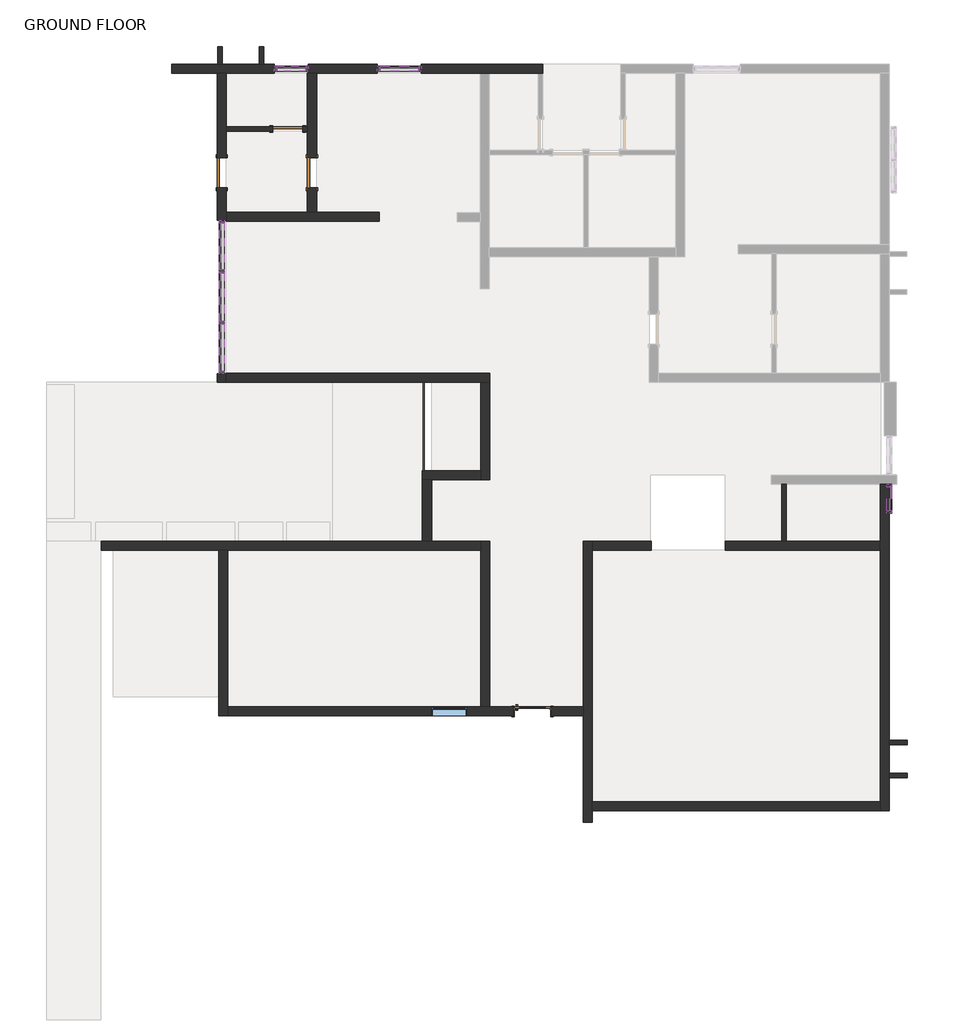
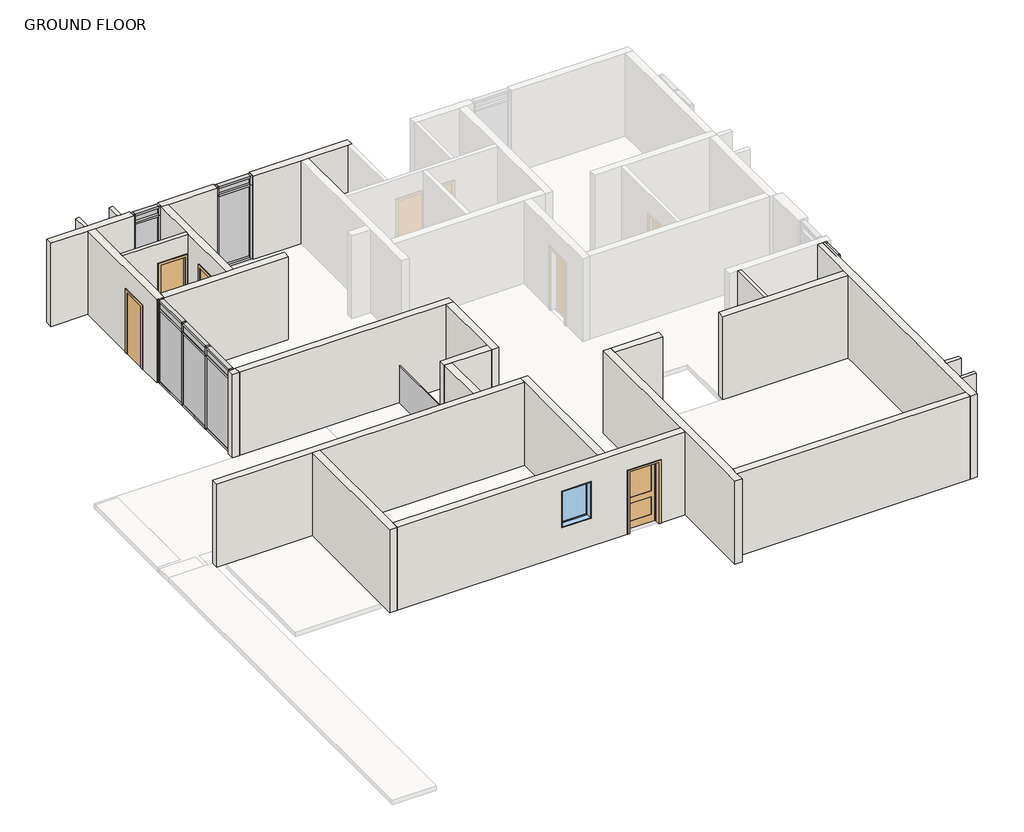
# One storey, part 1 of 2: 38 members, 23 walls, 13 plates, 4 doors, 1 window.
"""IFC4 building model written with IfcOpenShell, lengths in millimetres."""

from ifc_helpers import new_model, si_unit, frame, origin, place, context, project, spatial, polyline, outline, extrude, faceted_brep, transform, mapped, element, save
from components import door_18b56f29, door_f2b275c1, door_85036156, member_3e1bda4a, member_b6df92ca, member_34ede31c, member_a972b4dd, member_f0fea5a5, member_75d1e245, member_ee409385, member_3c3dc66a, member_8f63b531, member_3b0b2d0d, member_d7af48b5, member_8ca7f02a, member_47bfaf8a, member_6e77e263, system_panel_glazed_33731b62, system_panel_glazed_44b51bf5, system_panel_glazed_4e629a68, system_panel_glazed_8059ee36, system_panel_glazed_a992b757, system_panel_glazed_7419534f, system_panel_glazed_091cc013, system_panel_glazed_6c905176, system_panel_glazed_bc4b8a1a, system_panel_glazed_9fd37d83, system_panel_glazed_bf88fd99, window_c1f32544

model = new_model("IFC4")

# Units and contexts
model_context = context("Model", 3, world=origin())
ifc_project = project(units=[si_unit("LENGTHUNIT", "METRE", prefix="MILLI")], contexts=[model_context])

# Site, building, storey
site = spatial("IfcSite", under=ifc_project)
building = spatial("IfcBuilding", under=site)
storey = spatial("IfcBuildingStorey", under=building, Name="GROUND FLOOR", Elevation=304.8)

# Doors
placement = place(None, origin())
door_shape = door_18b56f29(model_context)
element("IfcDoor", 1, ObjectType="Door-Interior-Single-2_Panel-Wood : 36\" x 80\"", at=placement, inside=storey, context=model_context, shape_type="MappedRepresentation", body=[
    mapped(door_shape, transform((2388.7237558, 174.0966143, 304.8), x_axis=(1.0, 0.0, 0.0), y_axis=(0.0, 1.0, 0.0), z_axis=(0.0, 0.0, 1.0))),
])
door_2_shape = door_f2b275c1(model_context)
element("IfcDoor", 2, ObjectType="Single-Flush : 30\" x 80\"", at=placement, inside=storey, context=model_context, shape_type="MappedRepresentation", body=[
    mapped(door_2_shape, transform((-3801.944009, 14911.54348, 304.8), x_axis=(-1.0, 0.0, 0.0), y_axis=(0.0, -1.0, 0.0), z_axis=(0.0, 0.0, 1.0))),
])
door_3_shape = door_85036156(model_context)
element("IfcDoor", 3, ObjectType="Single-Flush : 30\" x 80\"", at=placement, inside=storey, context=model_context, shape_type="MappedRepresentation", body=[
    mapped(door_3_shape, transform((-3192.344009, 13803.0266219, 304.8), x_axis=(0.0, -1.0, 0.0), y_axis=(1.0, 0.0, 0.0), z_axis=(0.0, 0.0, 1.0))),
])
element("IfcDoor", 4, ObjectType="Single-Flush : 30\" x 80\"", at=placement, inside=storey, context=model_context, shape_type="MappedRepresentation", body=[
    mapped(door_3_shape, transform((-5478.344009, 13803.0266219, 304.8), x_axis=(0.0, -1.0, 0.0), y_axis=(1.0, 0.0, 0.0), z_axis=(0.0, 0.0, 1.0))),
])

# Members
member_shape = member_3e1bda4a(model_context)
element("IfcMember", 5, ObjectType="Rectangular Mullion : 2.5\" x 5\" rectangular", at=placement, inside=storey, context=model_context, shape_type="MappedRepresentation", body=[
    mapped(member_shape, transform((-5478.344009, 12544.7356247, 3048.0), x_axis=(0.0, 0.0, 1.0), y_axis=(1.0, 0.0, 0.0), z_axis=(0.0, 1.0, 0.0))),
])
element("IfcMember", 6, ObjectType="Rectangular Mullion : 2.5\" x 5\" rectangular", at=placement, inside=storey, context=model_context, shape_type="MappedRepresentation", body=[
    mapped(member_shape, transform((-5478.344009, 9985.6856249, 3048.0), x_axis=(0.0, 0.0, 1.0), y_axis=(1.0, 0.0, 0.0), z_axis=(0.0, 1.0, 0.0))),
])
member_2_shape = member_b6df92ca(model_context)
element("IfcMember", 7, ObjectType="Rectangular Mullion : 2.5\" x 5\" rectangular", at=placement, inside=storey, context=model_context, shape_type="MappedRepresentation", body=[
    mapped(member_2_shape, transform((-5478.344009, 11281.0856246, 3048.0), x_axis=(0.0, 0.0, 1.0), y_axis=(1.0, 0.0, 0.0), z_axis=(0.0, 1.0, 0.0))),
])
element("IfcMember", 8, ObjectType="Rectangular Mullion : 2.5\" x 5\" rectangular", at=placement, inside=storey, context=model_context, shape_type="MappedRepresentation", body=[
    mapped(member_shape, transform((-5478.344009, 8785.5356247, 304.8), x_axis=(0.0, 0.0, -1.0), y_axis=(1.0, 0.0, 0.0), z_axis=(0.0, -1.0, 0.0))),
])
element("IfcMember", 9, ObjectType="Rectangular Mullion : 2.5\" x 5\" rectangular", at=placement, inside=storey, context=model_context, shape_type="MappedRepresentation", body=[
    mapped(member_shape, transform((-5478.344009, 11344.5856246, 304.8), x_axis=(0.0, 0.0, -1.0), y_axis=(1.0, 0.0, 0.0), z_axis=(0.0, -1.0, 0.0))),
])
element("IfcMember", 10, ObjectType="Rectangular Mullion : 2.5\" x 5\" rectangular", at=placement, inside=storey, context=model_context, shape_type="MappedRepresentation", body=[
    mapped(member_2_shape, transform((-5478.344009, 10049.1856249, 304.8), x_axis=(0.0, 0.0, -1.0), y_axis=(1.0, 0.0, 0.0), z_axis=(0.0, -1.0, 0.0))),
])
member_3_shape = member_34ede31c(model_context)
element("IfcMember", 11, ObjectType="Rectangular Mullion : 2.5\" x 5\" rectangular", at=placement, inside=storey, context=model_context, shape_type="MappedRepresentation", body=[
    mapped(member_3_shape, transform((-5478.344009, 9985.6856249, 2743.2), x_axis=(0.0, 0.0, 1.0), y_axis=(1.0, 0.0, 0.0), z_axis=(0.0, 1.0, 0.0))),
])
element("IfcMember", 12, ObjectType="Rectangular Mullion : 2.5\" x 5\" rectangular", at=placement, inside=storey, context=model_context, shape_type="MappedRepresentation", body=[
    mapped(member_3_shape, transform((-5478.344009, 12544.7356247, 2743.2), x_axis=(0.0, 0.0, 1.0), y_axis=(1.0, 0.0, 0.0), z_axis=(0.0, 1.0, 0.0))),
])
member_4_shape = member_a972b4dd(model_context)
element("IfcMember", 13, ObjectType="Rectangular Mullion : 2.5\" x 5\" rectangular", at=placement, inside=storey, context=model_context, shape_type="MappedRepresentation", body=[
    mapped(member_4_shape, transform((-5478.344009, 11281.0856246, 2743.2), x_axis=(0.0, 0.0, 1.0), y_axis=(1.0, 0.0, 0.0), z_axis=(0.0, 1.0, 0.0))),
])
member_5_shape = member_f0fea5a5(model_context)
element("IfcMember", 14, ObjectType="Rectangular Mullion : 2.5\" x 5\" rectangular", at=placement, inside=storey, context=model_context, shape_type="MappedRepresentation", body=[
    mapped(member_5_shape, transform((-5478.344009, 10017.4356249, 304.8), x_axis=(0.0, 1.0, 0.0), y_axis=(1.0, 0.0, 0.0), z_axis=(0.0, 0.0, -1.0))),
])
element("IfcMember", 15, ObjectType="Rectangular Mullion : 2.5\" x 5\" rectangular", at=placement, inside=storey, context=model_context, shape_type="MappedRepresentation", body=[
    mapped(member_5_shape, transform((-5478.344009, 11312.8356246, 304.8), x_axis=(0.0, 1.0, 0.0), y_axis=(1.0, 0.0, 0.0), z_axis=(0.0, 0.0, -1.0))),
])
member_6_shape = member_75d1e245(model_context)
element("IfcMember", 16, ObjectType="Rectangular Mullion : 2.5\" x 5\" rectangular", at=placement, inside=storey, context=model_context, shape_type="MappedRepresentation", body=[
    mapped(member_6_shape, transform((-5478.344009, 10017.4356249, 2743.2), x_axis=(0.0, 1.0, 0.0), y_axis=(1.0, 0.0, 0.0), z_axis=(0.0, 0.0, -1.0))),
])
element("IfcMember", 17, ObjectType="Rectangular Mullion : 2.5\" x 5\" rectangular", at=placement, inside=storey, context=model_context, shape_type="MappedRepresentation", body=[
    mapped(member_6_shape, transform((-5478.344009, 11312.8356246, 2743.2), x_axis=(0.0, 1.0, 0.0), y_axis=(1.0, 0.0, 0.0), z_axis=(0.0, 0.0, -1.0))),
])
member_7_shape = member_ee409385(model_context)
element("IfcMember", 18, ObjectType="Rectangular Mullion : 2.5\" x 5\" rectangular", at=placement, inside=storey, context=model_context, shape_type="MappedRepresentation", body=[
    mapped(member_7_shape, transform((-5478.344009, 12608.2356247, 304.8), x_axis=(0.0, 1.0, 0.0), y_axis=(1.0, 0.0, 0.0), z_axis=(0.0, 0.0, -1.0))),
])
element("IfcMember", 19, ObjectType="Rectangular Mullion : 2.5\" x 5\" rectangular", at=placement, inside=storey, context=model_context, shape_type="MappedRepresentation", body=[
    mapped(member_7_shape, transform((-423.744009, 16441.89348, 304.8), x_axis=(1.0, 0.0, 0.0), y_axis=(0.0, -1.0, 0.0), z_axis=(0.0, 0.0, -1.0))),
])
element("IfcMember", 20, ObjectType="Rectangular Mullion : 2.5\" x 5\" rectangular", at=placement, inside=storey, context=model_context, shape_type="MappedRepresentation", body=[
    mapped(member_7_shape, transform((-3281.244009, 16441.89348, 304.8), x_axis=(1.0, 0.0, 0.0), y_axis=(0.0, -1.0, 0.0), z_axis=(0.0, 0.0, -1.0))),
])
element("IfcMember", 21, ObjectType="Rectangular Mullion : 2.5\" x 5\" rectangular", at=placement, inside=storey, context=model_context, shape_type="MappedRepresentation", body=[
    mapped(member_7_shape, transform((11414.0141504, 5181.56982, 304.8), x_axis=(0.0, -1.0, 0.0), y_axis=(-1.0, 0.0, 0.0), z_axis=(0.0, 0.0, -1.0))),
])
member_8_shape = member_3c3dc66a(model_context)
element("IfcMember", 22, ObjectType="Rectangular Mullion : 2.5\" x 5\" rectangular", at=placement, inside=storey, context=model_context, shape_type="MappedRepresentation", body=[
    mapped(member_8_shape, transform((-5478.344009, 12608.2356247, 2743.2), x_axis=(0.0, 1.0, 0.0), y_axis=(1.0, 0.0, 0.0), z_axis=(0.0, 0.0, -1.0))),
])
element("IfcMember", 23, ObjectType="Rectangular Mullion : 2.5\" x 5\" rectangular", at=placement, inside=storey, context=model_context, shape_type="MappedRepresentation", body=[
    mapped(member_8_shape, transform((-423.744009, 16441.89348, 2743.2), x_axis=(1.0, 0.0, 0.0), y_axis=(0.0, -1.0, 0.0), z_axis=(0.0, 0.0, -1.0))),
])
element("IfcMember", 24, ObjectType="Rectangular Mullion : 2.5\" x 5\" rectangular", at=placement, inside=storey, context=model_context, shape_type="MappedRepresentation", body=[
    mapped(member_8_shape, transform((-3281.244009, 16441.89348, 2743.2), x_axis=(1.0, 0.0, 0.0), y_axis=(0.0, -1.0, 0.0), z_axis=(0.0, 0.0, -1.0))),
])
element("IfcMember", 25, ObjectType="Rectangular Mullion : 2.5\" x 5\" rectangular", at=placement, inside=storey, context=model_context, shape_type="MappedRepresentation", body=[
    mapped(member_8_shape, transform((11414.0141504, 5181.56982, 2743.2), x_axis=(0.0, -1.0, 0.0), y_axis=(-1.0, 0.0, 0.0), z_axis=(0.0, 0.0, -1.0))),
])
element("IfcMember", 26, ObjectType="Rectangular Mullion : 2.5\" x 5\" rectangular", at=placement, inside=storey, context=model_context, shape_type="MappedRepresentation", body=[
    mapped(member_8_shape, transform((-5478.344009, 8722.0356247, 3048.0), x_axis=(0.0, -1.0, 0.0), y_axis=(1.0, 0.0, 0.0), z_axis=(0.0, 0.0, 1.0))),
])
element("IfcMember", 27, ObjectType="Rectangular Mullion : 2.5\" x 5\" rectangular", at=placement, inside=storey, context=model_context, shape_type="MappedRepresentation", body=[
    mapped(member_8_shape, transform((-1541.344009, 16441.89348, 3048.0), x_axis=(-1.0, 0.0, 0.0), y_axis=(0.0, -1.0, 0.0), z_axis=(0.0, 0.0, 1.0))),
])
element("IfcMember", 28, ObjectType="Rectangular Mullion : 2.5\" x 5\" rectangular", at=placement, inside=storey, context=model_context, shape_type="MappedRepresentation", body=[
    mapped(member_8_shape, transform((-4144.844009, 16441.89348, 3048.0), x_axis=(-1.0, 0.0, 0.0), y_axis=(0.0, -1.0, 0.0), z_axis=(0.0, 0.0, 1.0))),
])
element("IfcMember", 29, ObjectType="Rectangular Mullion : 2.5\" x 5\" rectangular", at=placement, inside=storey, context=model_context, shape_type="MappedRepresentation", body=[
    mapped(member_8_shape, transform((11414.0141504, 5918.16982, 3048.0), x_axis=(0.0, 1.0, 0.0), y_axis=(-1.0, 0.0, 0.0), z_axis=(0.0, 0.0, 1.0))),
])
element("IfcMember", 30, ObjectType="Rectangular Mullion : 2.5\" x 5\" rectangular", at=placement, inside=storey, context=model_context, shape_type="MappedRepresentation", body=[
    mapped(member_7_shape, transform((-5478.344009, 8722.0356247, 2743.2), x_axis=(0.0, -1.0, 0.0), y_axis=(1.0, 0.0, 0.0), z_axis=(0.0, 0.0, 1.0))),
])
element("IfcMember", 31, ObjectType="Rectangular Mullion : 2.5\" x 5\" rectangular", at=placement, inside=storey, context=model_context, shape_type="MappedRepresentation", body=[
    mapped(member_7_shape, transform((-1541.344009, 16441.89348, 2743.2), x_axis=(-1.0, 0.0, 0.0), y_axis=(0.0, -1.0, 0.0), z_axis=(0.0, 0.0, 1.0))),
])
element("IfcMember", 32, ObjectType="Rectangular Mullion : 2.5\" x 5\" rectangular", at=placement, inside=storey, context=model_context, shape_type="MappedRepresentation", body=[
    mapped(member_7_shape, transform((-4144.844009, 16441.89348, 2743.2), x_axis=(-1.0, 0.0, 0.0), y_axis=(0.0, -1.0, 0.0), z_axis=(0.0, 0.0, 1.0))),
])
element("IfcMember", 33, ObjectType="Rectangular Mullion : 2.5\" x 5\" rectangular", at=placement, inside=storey, context=model_context, shape_type="MappedRepresentation", body=[
    mapped(member_7_shape, transform((11414.0141504, 5918.16982, 2743.2), x_axis=(0.0, 1.0, 0.0), y_axis=(-1.0, 0.0, 0.0), z_axis=(0.0, 0.0, 1.0))),
])
member_9_shape = member_8f63b531(model_context)
element("IfcMember", 34, ObjectType="Rectangular Mullion : 2.5\" x 5\" rectangular", at=placement, inside=storey, context=model_context, shape_type="MappedRepresentation", body=[
    mapped(member_9_shape, transform((-487.244009, 16441.89348, 3048.0), x_axis=(0.0, 0.0, 1.0), y_axis=(0.0, -1.0, 0.0), z_axis=(1.0, 0.0, 0.0))),
])
element("IfcMember", 35, ObjectType="Rectangular Mullion : 2.5\" x 5\" rectangular", at=placement, inside=storey, context=model_context, shape_type="MappedRepresentation", body=[
    mapped(member_9_shape, transform((-1477.844009, 16441.89348, 304.8), x_axis=(0.0, 0.0, -1.0), y_axis=(0.0, -1.0, 0.0), z_axis=(-1.0, 0.0, 0.0))),
])
member_10_shape = member_3b0b2d0d(model_context)
element("IfcMember", 36, ObjectType="Rectangular Mullion : 2.5\" x 5\" rectangular", at=placement, inside=storey, context=model_context, shape_type="MappedRepresentation", body=[
    mapped(member_10_shape, transform((-487.244009, 16441.89348, 2743.2), x_axis=(0.0, 0.0, 1.0), y_axis=(0.0, -1.0, 0.0), z_axis=(1.0, 0.0, 0.0))),
])
member_11_shape = member_d7af48b5(model_context)
element("IfcMember", 37, ObjectType="Rectangular Mullion : 2.5\" x 5\" rectangular", at=placement, inside=storey, context=model_context, shape_type="MappedRepresentation", body=[
    mapped(member_11_shape, transform((-3344.744009, 16441.89348, 3048.0), x_axis=(0.0, 0.0, 1.0), y_axis=(0.0, -1.0, 0.0), z_axis=(1.0, 0.0, 0.0))),
])
element("IfcMember", 38, ObjectType="Rectangular Mullion : 2.5\" x 5\" rectangular", at=placement, inside=storey, context=model_context, shape_type="MappedRepresentation", body=[
    mapped(member_11_shape, transform((-4081.344009, 16441.89348, 304.8), x_axis=(0.0, 0.0, -1.0), y_axis=(0.0, -1.0, 0.0), z_axis=(-1.0, 0.0, 0.0))),
])
member_12_shape = member_8ca7f02a(model_context)
element("IfcMember", 39, ObjectType="Rectangular Mullion : 2.5\" x 5\" rectangular", at=placement, inside=storey, context=model_context, shape_type="MappedRepresentation", body=[
    mapped(member_12_shape, transform((-3344.744009, 16441.89348, 2743.2), x_axis=(0.0, 0.0, 1.0), y_axis=(0.0, -1.0, 0.0), z_axis=(1.0, 0.0, 0.0))),
])
member_13_shape = member_47bfaf8a(model_context)
element("IfcMember", 40, ObjectType="Rectangular Mullion : 2.5\" x 5\" rectangular", at=placement, inside=storey, context=model_context, shape_type="MappedRepresentation", body=[
    mapped(member_13_shape, transform((11414.0141504, 5245.06982, 3048.0), x_axis=(0.0, 0.0, 1.0), y_axis=(-1.0, 0.0, 0.0), z_axis=(0.0, -1.0, 0.0))),
])
element("IfcMember", 41, ObjectType="Rectangular Mullion : 2.5\" x 5\" rectangular", at=placement, inside=storey, context=model_context, shape_type="MappedRepresentation", body=[
    mapped(member_13_shape, transform((11414.0141504, 5854.66982, 304.8), x_axis=(0.0, 0.0, -1.0), y_axis=(-1.0, 0.0, 0.0), z_axis=(0.0, 1.0, 0.0))),
])
member_14_shape = member_6e77e263(model_context)
element("IfcMember", 42, ObjectType="Rectangular Mullion : 2.5\" x 5\" rectangular", at=placement, inside=storey, context=model_context, shape_type="MappedRepresentation", body=[
    mapped(member_14_shape, transform((11414.0141504, 5245.06982, 2743.2), x_axis=(0.0, 0.0, 1.0), y_axis=(-1.0, 0.0, 0.0), z_axis=(0.0, -1.0, 0.0))),
])

# Plates
system_panel_glazed_shape = system_panel_glazed_33731b62(model_context)
element("IfcPlate", 43, ObjectType="System Panel : Glazed", at=placement, inside=storey, context=model_context, shape_type="MappedRepresentation", body=[
    mapped(system_panel_glazed_shape, transform((-5478.344009, 9385.6106248, 368.3), x_axis=(0.0, 1.0, 0.0), y_axis=(-1.0, 0.0, 0.0), z_axis=(0.0, 0.0, 1.0))),
])
element("IfcPlate", 44, ObjectType="System Panel : Glazed", at=placement, inside=storey, context=model_context, shape_type="MappedRepresentation", body=[
    mapped(system_panel_glazed_shape, transform((-5478.344009, 11944.6606247, 368.3), x_axis=(0.0, 1.0, 0.0), y_axis=(-1.0, 0.0, 0.0), z_axis=(0.0, 0.0, 1.0))),
])
system_panel_glazed_2_shape = system_panel_glazed_44b51bf5(model_context)
element("IfcPlate", 45, ObjectType="System Panel : Glazed", at=placement, inside=storey, context=model_context, shape_type="MappedRepresentation", body=[
    mapped(system_panel_glazed_2_shape, transform((-5478.344009, 10665.1356247, 368.3), x_axis=(0.0, 1.0, 0.0), y_axis=(-1.0, 0.0, 0.0), z_axis=(0.0, 0.0, 1.0))),
])
system_panel_glazed_3_shape = system_panel_glazed_4e629a68(model_context)
element("IfcPlate", 46, ObjectType="System Panel : Glazed", at=placement, inside=storey, context=model_context, shape_type="MappedRepresentation", body=[
    mapped(system_panel_glazed_3_shape, transform((-5478.344009, 9385.6106248, 2774.95), x_axis=(0.0, 1.0, 0.0), y_axis=(-1.0, 0.0, 0.0), z_axis=(0.0, 0.0, 1.0))),
])
element("IfcPlate", 47, ObjectType="System Panel : Glazed", at=placement, inside=storey, context=model_context, shape_type="MappedRepresentation", body=[
    mapped(system_panel_glazed_3_shape, transform((-5478.344009, 11944.6606247, 2774.95), x_axis=(0.0, 1.0, 0.0), y_axis=(-1.0, 0.0, 0.0), z_axis=(0.0, 0.0, 1.0))),
])
system_panel_glazed_4_shape = system_panel_glazed_8059ee36(model_context)
element("IfcPlate", 48, ObjectType="System Panel : Glazed", at=placement, inside=storey, context=model_context, shape_type="MappedRepresentation", body=[
    mapped(system_panel_glazed_4_shape, transform((-5478.344009, 10665.1356247, 2774.95), x_axis=(0.0, 1.0, 0.0), y_axis=(-1.0, 0.0, 0.0), z_axis=(0.0, 0.0, 1.0))),
])
system_panel_glazed_5_shape = system_panel_glazed_a992b757(model_context)
element("IfcPlate", 49, ObjectType="System Panel : Glazed", at=placement, inside=storey, context=model_context, shape_type="MappedRepresentation", body=[
    mapped(system_panel_glazed_5_shape, transform((-982.544009, 16441.89348, 368.3), x_axis=(1.0, 0.0, 0.0), y_axis=(0.0, 1.0, 0.0), z_axis=(0.0, 0.0, 1.0))),
])
system_panel_glazed_6_shape = system_panel_glazed_7419534f(model_context)
element("IfcPlate", 50, ObjectType="System Panel : Glazed", at=placement, inside=storey, context=model_context, shape_type="MappedRepresentation", body=[
    mapped(system_panel_glazed_6_shape, transform((-982.544009, 16441.89348, 2774.95), x_axis=(1.0, 0.0, 0.0), y_axis=(0.0, 1.0, 0.0), z_axis=(0.0, 0.0, 1.0))),
])
system_panel_glazed_7_shape = system_panel_glazed_091cc013(model_context)
element("IfcPlate", 51, ObjectType="System Panel : Glazed", at=placement, inside=storey, context=model_context, shape_type="MappedRepresentation", body=[
    mapped(system_panel_glazed_7_shape, transform((-3713.044009, 16441.89348, 368.3), x_axis=(1.0, 0.0, 0.0), y_axis=(0.0, 1.0, 0.0), z_axis=(0.0, 0.0, 1.0))),
])
system_panel_glazed_8_shape = system_panel_glazed_6c905176(model_context)
element("IfcPlate", 52, ObjectType="System Panel : Glazed", at=placement, inside=storey, context=model_context, shape_type="MappedRepresentation", body=[
    mapped(system_panel_glazed_8_shape, transform((-3713.044009, 16441.89348, 2774.95), x_axis=(1.0, 0.0, 0.0), y_axis=(0.0, 1.0, 0.0), z_axis=(0.0, 0.0, 1.0))),
])
system_panel_glazed_9_shape = system_panel_glazed_bc4b8a1a(model_context)
element("IfcPlate", 53, ObjectType="System Panel : Glazed", at=placement, inside=storey, context=model_context, shape_type="MappedRepresentation", body=[
    mapped(system_panel_glazed_9_shape, transform((11414.0141504, 5549.86982, 368.3), x_axis=(0.0, -1.0, 0.0), y_axis=(1.0, 0.0, 0.0), z_axis=(0.0, 0.0, 1.0))),
])
system_panel_glazed_10_shape = system_panel_glazed_9fd37d83(model_context)
element("IfcPlate", 54, ObjectType="System Panel : Glazed", at=placement, inside=storey, context=model_context, shape_type="MappedRepresentation", body=[
    mapped(system_panel_glazed_10_shape, transform((11414.0141504, 5549.86982, 2774.95), x_axis=(0.0, -1.0, 0.0), y_axis=(1.0, 0.0, 0.0), z_axis=(0.0, 0.0, 1.0))),
])
system_panel_glazed_11_shape = system_panel_glazed_bf88fd99(model_context)
element("IfcPlate", 55, ObjectType="System Panel : Glazed", at=placement, inside=storey, context=model_context, shape_type="MappedRepresentation", body=[
    mapped(system_panel_glazed_11_shape, transform((-396.2931047, 7382.1856247, 304.8), x_axis=(0.0, -1.0, 0.0), y_axis=(1.0, 0.0, 0.0), z_axis=(0.0, 0.0, 1.0))),
])

# Walls
element("IfcWall", 56, ObjectType="INNER WALL 4.5\"", at=placement, inside=storey, context=model_context, shape_type="SweptSolid", body=[
    extrude(outline(polyline([(304.8, -5364.044009), (304.8, -4182.944009), (2336.8, -4182.944009), (2336.8, -3420.944009), (304.8, -3420.944009), (304.8, -3306.644009), (3048.0, -3306.644009), (3048.0, -5364.044009), (304.8, -5364.044009)])), frame((0.0, 14854.39348, 0.0), z_axis=(0.0, 1.0, 0.0), x_axis=(0.0, 0.0, 1.0)), (0.0, 0.0, 1.0), 114.3),
])
element("IfcWall", 57, ObjectType="INNER WALL 4.5\"", at=placement, inside=storey, context=model_context, shape_type="SweptSolid", body=[
    extrude(outline(polyline([(11871.2141504, -670.6966507), (11414.0141504, -670.6966507), (11414.0141504, -556.3966507), (11871.2141504, -556.3966507), (11871.2141504, -670.6966507)])), frame((0.0, 0.0, 304.8), z_axis=(0.0, 0.0, 1.0), x_axis=(1.0, 0.0, 0.0)), (0.0, 0.0, 1.0), 2743.2),
])
element("IfcWall", 58, ObjectType="INNER WALL 4.5\"", at=placement, inside=storey, context=model_context, shape_type="SweptSolid", body=[
    extrude(outline(polyline([(11871.2141504, -1502.5466507), (11414.0141504, -1502.5466507), (11414.0141504, -1388.2466507), (11871.2141504, -1388.2466507), (11871.2141504, -1502.5466507)])), frame((0.0, 0.0, 304.8), z_axis=(0.0, 0.0, 1.0), x_axis=(1.0, 0.0, 0.0)), (0.0, 0.0, 1.0), 2743.2),
])
element("IfcWall", 59, ObjectType="INNER WALL 4.5\"", at=placement, inside=storey, context=model_context, shape_type="SweptSolid", body=[
    extrude(outline(polyline([(-5577.3305586, 16556.19348), (-5577.3305586, 17000.8847206), (-5463.0305586, 17000.8847206), (-5463.0305586, 16556.19348), (-5577.3305586, 16556.19348)])), frame((0.0, 0.0, 304.8), z_axis=(0.0, 0.0, 1.0), x_axis=(1.0, 0.0, 0.0)), (0.0, 0.0, 1.0), 2743.2),
])
element("IfcWall", 60, ObjectType="INNER WALL 4.5\"", at=placement, inside=storey, context=model_context, shape_type="SweptSolid", body=[
    extrude(outline(polyline([(-4532.194009, 16556.19348), (-4532.194009, 17000.8847206), (-4417.894009, 17000.8847206), (-4417.894009, 16556.19348), (-4532.194009, 16556.19348)])), frame((0.0, 0.0, 304.8), z_axis=(0.0, 0.0, 1.0), x_axis=(1.0, 0.0, 0.0)), (0.0, 0.0, 1.0), 2743.2),
])
element("IfcWall", 61, ObjectType="INNER WALL 4.5\"", at=placement, inside=storey, context=model_context, shape_type="SweptSolid", body=[
    extrude(outline(polyline([(8810.5141504, 5918.16982), (8810.5141504, 4478.232458), (8696.2141504, 4478.232458), (8696.2141504, 5918.16982), (8810.5141504, 5918.16982)])), frame((0.0, 0.0, 304.8), z_axis=(0.0, 0.0, 1.0), x_axis=(1.0, 0.0, 0.0)), (0.0, 0.0, 1.0), 2743.2),
])
element("IfcWall", 62, ObjectType="OUTER WALL THICKNESS 9\"", at=placement, inside=storey, context=model_context, shape_type="Brep", body=[
    faceted_brep([(-6748.344009, 16327.59348, 3048.0), (-6748.344009, 16327.59348, 304.8), (-5592.644009, 16327.59348, 304.8), (-5364.044009, 16327.59348, 304.8), (-4144.844009, 16327.59348, 304.8), (-4144.844009, 16327.59348, 3048.0), (-5364.044009, 16327.59348, 3048.0), (-5592.644009, 16327.59348, 3048.0), (-6748.344009, 16556.19348, 304.8), (-6748.344009, 16556.19348, 3048.0), (-5577.3305586, 16556.19348, 3048.0), (-5463.0305586, 16556.19348, 3048.0), (-4532.194009, 16556.19348, 3048.0), (-4417.894009, 16556.19348, 3048.0), (-4144.844009, 16556.19348, 3048.0), (-4144.844009, 16556.19348, 304.8), (-4417.894009, 16556.19348, 304.8), (-4532.194009, 16556.19348, 304.8), (-5463.0305586, 16556.19348, 304.8), (-5577.3305586, 16556.19348, 304.8)], [[[0, 1, 2, 3, 4, 5, 6, 7]], [[8, 9, 10, 11, 12, 13, 14, 15, 16, 17, 18, 19]], [[1, 8, 19, 18, 17, 16, 15, 4, 3, 2]], [[9, 0, 7, 6, 5, 14, 13, 12, 11, 10]], [[1, 0, 9, 8]], [[5, 4, 15, 14]]]),
    faceted_brep([(2649.655991, 16327.59348, 304.8), (2649.655991, 16327.59348, 3048.0), (2535.355991, 16327.59348, 3048.0), (1297.105991, 16327.59348, 3048.0), (1068.505991, 16327.59348, 3048.0), (-423.744009, 16327.59348, 3048.0), (-423.744009, 16327.59348, 304.8), (1068.505991, 16327.59348, 304.8), (1297.105991, 16327.59348, 304.8), (2535.355991, 16327.59348, 304.8), (2649.655991, 16556.19348, 3048.0), (2649.655991, 16556.19348, 304.8), (-423.744009, 16556.19348, 304.8), (-423.744009, 16556.19348, 3048.0)], [[[0, 1, 2, 3, 4, 5, 6, 7, 8, 9]], [[10, 11, 12, 13]], [[11, 0, 9, 8, 7, 6, 12]], [[1, 10, 13, 5, 4, 3, 2]], [[1, 0, 11, 10]], [[6, 5, 13, 12]]]),
    faceted_brep([(-1541.344009, 16327.59348, 304.8), (-1541.344009, 16327.59348, 3048.0), (-3078.044009, 16327.59348, 3048.0), (-3281.244009, 16327.59348, 3048.0), (-3281.244009, 16327.59348, 304.8), (-3078.044009, 16327.59348, 304.8), (-1541.344009, 16556.19348, 3048.0), (-1541.344009, 16556.19348, 304.8), (-3281.244009, 16556.19348, 304.8), (-3281.244009, 16556.19348, 3048.0)], [[[0, 1, 2, 3, 4, 5]], [[6, 7, 8, 9]], [[7, 0, 5, 4, 8]], [[1, 6, 9, 3, 2]], [[1, 0, 7, 6]], [[4, 3, 9, 8]]]),
])
element("IfcWall", 63, ObjectType="OUTER WALL THICKNESS 9\"", at=placement, inside=storey, context=model_context, shape_type="Brep", body=[
    faceted_brep([(-5592.644009, 8504.39348, 304.8), (-5592.644009, 8504.39348, 3048.0), (-5592.644009, 8722.0356247, 3048.0), (-5592.644009, 8722.0356247, 304.8), (-5364.044009, 8504.39348, 3048.0), (-5364.044009, 8504.39348, 304.8), (-5364.044009, 8506.1356247, 304.8), (-5364.044009, 8722.0356247, 304.8), (-5364.044009, 8722.0356247, 3048.0), (-5364.044009, 8506.1356247, 3048.0)], [[[0, 1, 2, 3]], [[4, 5, 6, 7, 8, 9]], [[5, 0, 3, 7, 6]], [[1, 0, 5, 4]], [[1, 4, 9, 8, 2]], [[3, 2, 8, 7]]]),
    faceted_brep([(-5592.644009, 16327.59348, 3048.0), (-5592.644009, 16327.59348, 304.8), (-5592.644009, 14184.0266219, 304.8), (-5592.644009, 14184.0266219, 2336.8), (-5592.644009, 13422.0266219, 2336.8), (-5592.644009, 13422.0266219, 304.8), (-5592.644009, 12608.2356247, 304.8), (-5592.644009, 12608.2356247, 3048.0), (-5364.044009, 16327.59348, 304.8), (-5364.044009, 16327.59348, 3048.0), (-5364.044009, 14968.69348, 3048.0), (-5364.044009, 14854.39348, 3048.0), (-5364.044009, 12808.8097639, 3048.0), (-5364.044009, 12608.2356247, 3048.0), (-5364.044009, 12608.2356247, 304.8), (-5364.044009, 12808.8097639, 304.8), (-5364.044009, 13422.0266219, 304.8), (-5364.044009, 13422.0266219, 2336.8), (-5364.044009, 14184.0266219, 2336.8), (-5364.044009, 14184.0266219, 304.8), (-5364.044009, 14854.39348, 304.8), (-5364.044009, 14968.69348, 304.8)], [[[0, 1, 2, 3, 4, 5, 6, 7]], [[8, 9, 10, 11, 12, 13, 14, 15, 16, 17, 18, 19, 20, 21]], [[1, 8, 21, 20, 19, 2]], [[5, 16, 15, 14, 6]], [[9, 0, 7, 13, 12, 11, 10]], [[1, 0, 9, 8]], [[17, 16, 5, 4]], [[18, 17, 4, 3]], [[19, 18, 3, 2]], [[7, 6, 14, 13]]]),
])
element("IfcWall", 64, ObjectType="OUTER WALL THICKNESS 9\"", at=placement, inside=storey, context=model_context, shape_type="Brep", body=[
    faceted_brep([(1305.5068953, 8734.7356247, 304.8), (-5364.044009, 8734.7356247, 304.8), (-5364.044009, 8734.7356247, 3048.0), (1305.5068953, 8734.7356247, 3048.0), (1305.5068953, 8506.1356247, 304.8), (1305.5068953, 8506.1356247, 3048.0), (1076.9068953, 8506.1356247, 3048.0), (-5364.044009, 8506.1356247, 3048.0), (-5364.044009, 8506.1356247, 304.8), (-396.2931047, 8506.1356247, 304.8), (-167.6931047, 8506.1356247, 304.8), (1076.9068953, 8506.1356247, 304.8)], [[[0, 1, 2, 3]], [[4, 5, 6, 7, 8, 9, 10, 11]], [[1, 0, 4, 11, 10, 9, 8]], [[3, 2, 7, 6, 5]], [[2, 1, 8, 7]], [[0, 3, 5, 4]]]),
])
element("IfcWall", 65, ObjectType="OUTER WALL THICKNESS 9\"", at=placement, inside=storey, context=model_context, shape_type="Brep", body=[
    faceted_brep([(1076.9068953, 8506.1356247, 304.8), (1076.9068953, 6258.2356247, 304.8), (1076.9068953, 6029.6356247, 304.8), (1076.9068953, 6029.6356247, 3048.0), (1076.9068953, 6258.2356247, 3048.0), (1076.9068953, 8506.1356247, 3048.0), (1305.5068953, 8506.1356247, 304.8), (1305.5068953, 8506.1356247, 3048.0), (1305.5068953, 6029.6356247, 3048.0), (1305.5068953, 6029.6356247, 304.8)], [[[0, 1, 2, 3, 4, 5]], [[6, 7, 8, 9]], [[2, 1, 0, 6, 9]], [[5, 4, 3, 8, 7]], [[0, 5, 7, 6]], [[3, 2, 9, 8]]]),
])
element("IfcWall", 66, ObjectType="OUTER WALL THICKNESS 9\"", at=placement, inside=storey, context=model_context, shape_type="Brep", body=[
    faceted_brep([(1076.9068953, 6258.2356247, 304.8), (-396.2931047, 6258.2356247, 304.8), (-396.2931047, 6258.2356247, 3048.0), (1076.9068953, 6258.2356247, 3048.0), (1076.9068953, 6029.6356247, 304.8), (1076.9068953, 6029.6356247, 3048.0), (-167.6931047, 6029.6356247, 3048.0), (-396.2931047, 6029.6356247, 3048.0), (-396.2931047, 6029.6356247, 304.8), (-167.6931047, 6029.6356247, 304.8)], [[[0, 1, 2, 3]], [[4, 5, 6, 7, 8, 9]], [[1, 0, 4, 9, 8]], [[3, 2, 7, 6, 5]], [[0, 3, 5, 4]], [[2, 1, 8, 7]]]),
])
element("IfcWall", 67, ObjectType="OUTER WALL THICKNESS 9\"", at=placement, inside=storey, context=model_context, shape_type="Brep", body=[
    faceted_brep([(-3306.644009, 13422.0266219, 2336.8), (-3306.644009, 13422.0266219, 304.8), (-3306.644009, 12808.8097639, 304.8), (-3306.644009, 12808.8097639, 3048.0), (-3306.644009, 14854.39348, 3048.0), (-3306.644009, 14968.69348, 3048.0), (-3306.644009, 16327.59348, 3048.0), (-3306.644009, 16327.59348, 304.8), (-3306.644009, 14968.69348, 304.8), (-3306.644009, 14854.39348, 304.8), (-3306.644009, 14184.0266219, 304.8), (-3306.644009, 14184.0266219, 2336.8), (-3078.044009, 12808.8097639, 304.8), (-3078.044009, 13422.0266219, 304.8), (-3078.044009, 13422.0266219, 2336.8), (-3078.044009, 14184.0266219, 2336.8), (-3078.044009, 14184.0266219, 304.8), (-3078.044009, 16327.59348, 304.8), (-3078.044009, 16327.59348, 3048.0), (-3078.044009, 12808.8097639, 3048.0)], [[[0, 1, 2, 3, 4, 5, 6, 7, 8, 9, 10, 11]], [[12, 13, 14, 15, 16, 17, 18, 19]], [[2, 1, 13, 12]], [[10, 9, 8, 7, 17, 16]], [[6, 5, 4, 3, 19, 18]], [[7, 6, 18, 17]], [[3, 2, 12, 19]], [[14, 13, 1, 0]], [[15, 14, 0, 11]], [[16, 15, 11, 10]]]),
])
element("IfcWall", 68, ObjectType="OUTER WALL THICKNESS 9\"", at=placement, inside=storey, context=model_context, shape_type="Brep", body=[
    faceted_brep([(-1493.8979576, 12808.8097639, 304.8), (-3078.044009, 12808.8097639, 304.8), (-3306.644009, 12808.8097639, 304.8), (-5364.044009, 12808.8097639, 304.8), (-5364.044009, 12808.8097639, 3048.0), (-3306.644009, 12808.8097639, 3048.0), (-3078.044009, 12808.8097639, 3048.0), (-1493.8979576, 12808.8097639, 3048.0), (-1493.8979576, 12580.2097639, 304.8), (-1493.8979576, 12580.2097639, 3048.0), (-5364.044009, 12580.2097639, 3048.0), (-5364.044009, 12580.2097639, 304.8)], [[[0, 1, 2, 3, 4, 5, 6, 7]], [[8, 9, 10, 11]], [[3, 2, 1, 0, 8, 11]], [[7, 6, 5, 4, 10, 9]], [[0, 7, 9, 8]], [[4, 3, 11, 10]]]),
])
element("IfcWall", 69, ObjectType="OUTER WALL THICKNESS 9\"", at=placement, inside=storey, context=model_context, shape_type="Brep", body=[
    faceted_brep([(-5326.5262442, 56.6216143, 3048.0), (-5326.5262442, 56.6216143, 304.8), (-5326.5262442, 285.2216143, 304.8), (-5326.5262442, 4247.6216143, 304.8), (-5326.5262442, 4247.6216143, 3048.0), (-5326.5262442, 285.2216143, 3048.0), (-5555.1262442, 56.6216143, 304.8), (-5555.1262442, 56.6216143, 3048.0), (-5555.1262442, 4247.6216143, 3048.0), (-5555.1262442, 4247.6216143, 304.8)], [[[0, 1, 2, 3, 4, 5]], [[6, 7, 8, 9]], [[3, 2, 1, 6, 9]], [[0, 5, 4, 8, 7]], [[4, 3, 9, 8]], [[0, 7, 6, 1]]]),
])
element("IfcWall", 70, ObjectType="OUTER WALL THICKNESS 9\"", at=placement, inside=storey, context=model_context, shape_type="Brep", body=[
    faceted_brep([(3668.6367729, 56.6216143, 3048.0), (-5326.5262442, 56.6216143, 3048.0), (-5326.5262442, 56.6216143, 304.8), (1906.1237558, 56.6216143, 304.8), (1906.1237558, 56.6216143, 2362.2), (2871.3237558, 56.6216143, 2362.2), (2871.3237558, 56.6216143, 304.8), (3668.6367729, 56.6216143, 304.8), (737.7237558, 56.6216143, 2438.4), (737.7237558, 56.6216143, 1219.2), (-176.6762442, 56.6216143, 1219.2), (-176.6762442, 56.6216143, 2438.4), (-5326.5262442, 285.2216143, 3048.0), (1080.6237558, 285.2216143, 3048.0), (1309.2237558, 285.2216143, 3048.0), (3668.6367729, 285.2216143, 3048.0), (3668.6367729, 285.2216143, 304.8), (2871.3237558, 285.2216143, 304.8), (2871.3237558, 285.2216143, 2362.2), (1906.1237558, 285.2216143, 2362.2), (1906.1237558, 285.2216143, 304.8), (1309.2237558, 285.2216143, 304.8), (1080.6237558, 285.2216143, 304.8), (-5326.5262442, 285.2216143, 304.8), (737.7237558, 285.2216143, 2438.4), (-176.6762442, 285.2216143, 2438.4), (-176.6762442, 285.2216143, 1219.2), (737.7237558, 285.2216143, 1219.2)], [[[0, 1, 2, 3, 4, 5, 6, 7], [8, 9, 10, 11]], [[12, 13, 14, 15, 16, 17, 18, 19, 20, 21, 22, 23], [24, 25, 26, 27]], [[2, 23, 22, 21, 20, 3]], [[16, 7, 6, 17]], [[1, 0, 15, 14, 13, 12]], [[2, 1, 12, 23]], [[0, 7, 16, 15]], [[5, 18, 17, 6]], [[18, 5, 4, 19]], [[19, 4, 3, 20]], [[9, 8, 24, 27]], [[10, 9, 27, 26]], [[11, 10, 26, 25]], [[8, 11, 25, 24]]]),
])
element("IfcWall", 71, ObjectType="OUTER WALL THICKNESS 9\"", at=placement, inside=storey, context=model_context, shape_type="Brep", body=[
    faceted_brep([(1309.2237558, 285.2216143, 304.8), (1309.2237558, 4476.2216143, 304.8), (1309.2237558, 4476.2216143, 3048.0), (1309.2237558, 285.2216143, 3048.0), (1080.6237558, 285.2216143, 304.8), (1080.6237558, 285.2216143, 3048.0), (1080.6237558, 4247.6216143, 3048.0), (1080.6237558, 4476.2216143, 3048.0), (1080.6237558, 4476.2216143, 304.8), (1080.6237558, 4247.6216143, 304.8)], [[[0, 1, 2, 3]], [[4, 5, 6, 7, 8, 9]], [[1, 0, 4, 9, 8]], [[3, 2, 7, 6, 5]], [[0, 3, 5, 4]], [[2, 1, 8, 7]]]),
])
element("IfcWall", 72, ObjectType="OUTER WALL THICKNESS 9\"", at=placement, inside=storey, context=model_context, shape_type="Brep", body=[
    faceted_brep([(1080.6237558, 4476.2216143, 304.8), (-167.6931047, 4476.2216143, 304.8), (-396.2931047, 4476.2216143, 304.8), (-8533.2762442, 4476.2216143, 304.8), (-8533.2762442, 4476.2216143, 3048.0), (-396.2931047, 4476.2216143, 3048.0), (-167.6931047, 4476.2216143, 3048.0), (1080.6237558, 4476.2216143, 3048.0), (1080.6237558, 4247.6216143, 304.8), (1080.6237558, 4247.6216143, 3048.0), (-5326.5262442, 4247.6216143, 3048.0), (-5555.1262442, 4247.6216143, 3048.0), (-8533.2762442, 4247.6216143, 3048.0), (-8533.2762442, 4247.6216143, 1219.2), (-8533.2762442, 4247.6216143, 304.8), (-5555.1262442, 4247.6216143, 304.8), (-5326.5262442, 4247.6216143, 304.8)], [[[0, 1, 2, 3, 4, 5, 6, 7]], [[8, 9, 10, 11, 12, 13, 14, 15, 16]], [[3, 2, 1, 0, 8, 16, 15, 14]], [[7, 6, 5, 4, 12, 11, 10, 9]], [[0, 7, 9, 8]], [[4, 3, 14, 13, 12]]]),
])
element("IfcWall", 73, ObjectType="OUTER WALL THICKNESS 9\"", at=placement, inside=storey, context=model_context, shape_type="SweptSolid", body=[
    extrude(outline(polyline([(-396.2931047, 4476.2216143), (-396.2931047, 6029.6356247), (-167.6931047, 6029.6356247), (-167.6931047, 4476.2216143), (-396.2931047, 4476.2216143)])), frame((0.0, 0.0, 304.8), z_axis=(0.0, 0.0, 1.0), x_axis=(1.0, 0.0, 0.0)), (0.0, 0.0, 1.0), 2743.2),
])
element("IfcWall", 74, ObjectType="OUTER WALL THICKNESS 9\"", at=placement, inside=storey, context=model_context, shape_type="Brep", body=[
    faceted_brep([(11414.0141504, -2348.017542, 304.8), (11414.0141504, -1502.5466507, 304.8), (11414.0141504, -1388.2466507, 304.8), (11414.0141504, -670.6966507, 304.8), (11414.0141504, -556.3966507, 304.8), (11414.0141504, 5918.16982, 304.8), (11414.0141504, 5918.16982, 3048.0), (11414.0141504, -556.3966507, 3048.0), (11414.0141504, -670.6966507, 3048.0), (11414.0141504, -1388.2466507, 3048.0), (11414.0141504, -1502.5466507, 3048.0), (11414.0141504, -2348.017542, 3048.0), (11185.4141504, -2348.017542, 304.8), (11185.4141504, -2348.017542, 3048.0), (11185.4141504, -2119.417542, 3048.0), (11185.4141504, 4249.632458, 3048.0), (11185.4141504, 4478.232458, 3048.0), (11185.4141504, 5918.16982, 3048.0), (11185.4141504, 5918.16982, 304.8), (11185.4141504, 4478.232458, 304.8), (11185.4141504, 4249.632458, 304.8), (11185.4141504, -2119.417542, 304.8)], [[[0, 1, 2, 3, 4, 5, 6, 7, 8, 9, 10, 11]], [[12, 13, 14, 15, 16, 17, 18, 19, 20, 21]], [[5, 4, 3, 2, 1, 0, 12, 21, 20, 19, 18]], [[11, 10, 9, 8, 7, 6, 17, 16, 15, 14, 13]], [[6, 5, 18, 17]], [[0, 11, 13, 12]]]),
])
element("IfcWall", 75, ObjectType="OUTER WALL THICKNESS 9\"", at=placement, inside=storey, context=model_context, shape_type="Brep", body=[
    faceted_brep([(11185.4141504, 4478.232458, 304.8), (8810.5141504, 4478.232458, 304.8), (8696.2141504, 4478.232458, 304.8), (7273.8141504, 4478.232458, 304.8), (7273.8141504, 4478.232458, 3048.0), (8696.2141504, 4478.232458, 3048.0), (8810.5141504, 4478.232458, 3048.0), (11185.4141504, 4478.232458, 3048.0), (11185.4141504, 4249.632458, 304.8), (11185.4141504, 4249.632458, 3048.0), (7273.8141504, 4249.632458, 3048.0), (7273.8141504, 4249.632458, 304.8)], [[[0, 1, 2, 3, 4, 5, 6, 7]], [[8, 9, 10, 11]], [[3, 2, 1, 0, 8, 11]], [[4, 3, 11, 10]], [[7, 6, 5, 4, 10, 9]], [[0, 7, 9, 8]]]),
])
element("IfcWall", 76, ObjectType="OUTER WALL THICKNESS 9\"", at=placement, inside=storey, context=model_context, shape_type="Brep", body=[
    faceted_brep([(3668.6367729, 4478.232458, 304.8), (3668.6367729, 285.2216143, 304.8), (3668.6367729, 56.6216143, 304.8), (3668.6367729, -2635.5540506, 304.8), (3668.6367729, -2635.5540506, 3048.0), (3668.6367729, 56.6216143, 3048.0), (3668.6367729, 285.2216143, 3048.0), (3668.6367729, 4478.232458, 3048.0), (3897.2367729, 4478.232458, 304.8), (3897.2367729, 4478.232458, 3048.0), (3897.2367729, 4249.632458, 3048.0), (3897.2367729, -2119.417542, 3048.0), (3897.2367729, -2348.017542, 3048.0), (3897.2367729, -2635.5540506, 3048.0), (3897.2367729, -2635.5540506, 304.8), (3897.2367729, -2348.017542, 304.8), (3897.2367729, -2119.417542, 304.8), (3897.2367729, 4249.632458, 304.8)], [[[0, 1, 2, 3, 4, 5, 6, 7]], [[8, 9, 10, 11, 12, 13, 14, 15, 16, 17]], [[3, 2, 1, 0, 8, 17, 16, 15, 14]], [[4, 3, 14, 13]], [[7, 6, 5, 4, 13, 12, 11, 10, 9]], [[0, 7, 9, 8]]]),
])
element("IfcWall", 77, ObjectType="OUTER WALL THICKNESS 9\"", at=placement, inside=storey, context=model_context, shape_type="SweptSolid", body=[
    extrude(outline(polyline([(3897.2367729, -2119.417542), (11185.4141504, -2119.417542), (11185.4141504, -2348.017542), (3897.2367729, -2348.017542), (3897.2367729, -2119.417542)])), frame((0.0, 0.0, 304.8), z_axis=(0.0, 0.0, 1.0), x_axis=(1.0, 0.0, 0.0)), (0.0, 0.0, 1.0), 2743.2),
])
element("IfcWall", 78, ObjectType="OUTER WALL THICKNESS 9\"", at=placement, inside=storey, context=model_context, shape_type="SweptSolid", body=[
    extrude(outline(polyline([(5395.8367729, 4249.632458), (3897.2367729, 4249.632458), (3897.2367729, 4478.232458), (5395.8367729, 4478.232458), (5395.8367729, 4249.632458)])), frame((0.0, 0.0, 304.8), z_axis=(0.0, 0.0, 1.0), x_axis=(1.0, 0.0, 0.0)), (0.0, 0.0, 1.0), 2743.2),
])

# Window
window_shape = window_c1f32544(model_context)
element("IfcWindow", 79, ObjectType="Fixed : 36\" x 48\"", at=placement, inside=storey, context=model_context, shape_type="MappedRepresentation", body=[
    mapped(window_shape, transform((318.6237558, 170.9216143, 304.8), x_axis=(1.0, 0.0, 0.0), y_axis=(0.0, 1.0, 0.0), z_axis=(0.0, 0.0, 1.0))),
])

save(model, "model.ifc")

# Revit data of these elements
# Type "Door-Interior-Single-2_Panel-Wood : 36\" x 80\""
#   Type Mark = "8"
#   Assembly Code = "C1020300"
#   Analytic Construction = "Wooden"
#   Top Rail = 0' - 4 11/16"
#   Thickness = 0' - 1 3/8"
#   Thermal Resistance (R) = 2.5876 (h·ft²·°F)/BTU
#   Swing Angle [instance default] = 90.00°
#   Stiles = 0' - 4 3/4"
#   Rough Width = 3' - 2"
#   Rough Height = 6' - 9"
#   Lock Rail = 0' - 7 1/2"
#   Height = 6' - 8"
#   Width = 3' - 0"
#   Heat Transfer Coefficient (U) = 0.3865 BTU/(h·ft²·°F)
#   Bottom Rail = 0' - 9 1/8"
#   Trim Material = Cherry
#   Panel Material = Cherry
#   Frame Material = Cherry
#   Door Handle Material = Aluminum
#   Visual Light Transmittance = 0
#   Solar Heat Gain Coefficient = 0
#   Wall Closure = (empty or 0)
#   Function = (empty or 0)
# Type "Single-Flush : 30\" x 80\""
#   Type Mark = "5"
#   Construction Type Id = "MDOOR"
#   Assembly Code = "C1020"
#   Analytic Construction = "Metal"
#   Thickness = 0' - 2"
#   Heat Transfer Coefficient (U) = 0.651978 BTU/(h·ft²·°F)
#   Height = 6' - 8"
#   Trim Projection Ext = 0' - 1"
#   Trim Projection Int = 0' - 1"
#   Trim Width = 0' - 3"
#   Width = 2' - 6"
#   Define Thermal Properties by = 1
#   Define Thermal Properties by = 1
#   Door Material = Door - Panel
#   Frame Material = Door - Frame
#   Visual Light Transmittance = 0
#   Solar Heat Gain Coefficient = 0
#   Function = (empty or 0)
#   Wall Closure = (empty or 0)
# Type "Rectangular Mullion : 2.5\" x 5\" rectangular"
#   built-in parameter 1007304 = 0.416667 (stored number, unit not read)
#   built-in parameter 1007301 = 0.104167 (stored number, unit not read)
#   built-in parameter 1007300 = 0.104167 (stored number, unit not read)
# Type "System Panel : Glazed"
#   Construction Type Id = "GSP4R"
#   Analytic Construction = "1/8 in Pilkington single glazing"
#   Visual Light Transmittance = 0.9
#   Solar Heat Gain Coefficient = 0.86
#   Heat Transfer Coefficient (U) = 1.18115 BTU/(h·ft²·°F)
#   Define Thermal Properties by = 1
# Type "INNER WALL 4.5\""
#   Assembly Code = "B2010"
#   Layers, outside or top first: 0' - 4 1/2" "BEIGE COLOUR" (function 1)
# Type "OUTER WALL THICKNESS 9\""
#   Assembly Code = "B2010"
#   Layers, outside or top first: 0' - 9" "BEIGE COLOUR" (function 1)
# Type "Fixed : 36\" x 48\""
#   Type Mark = "1"
#   Construction Type Id = "GSP4R"
#   Assembly Code = "B2020100"
#   Analytic Construction = "1/8 in Pilkington single glazing"
#   Visual Light Transmittance = 0.9
#   Solar Heat Gain Coefficient = 0.78
#   Heat Transfer Coefficient (U) = 0.6496 BTU/(h·ft²·°F)
#   Height = 4' - 0"
#   Default Sill Height = 3' - 0"
#   Width = 3' - 0"
#   Window Inset = 0' - 0 3/4"
#   Define Thermal Properties by = 1
#   Define Thermal Properties by = 1
#   Glass Pane Material = Glass
#   Sash Material = Sash
#   Wall Closure = (empty or 0)
# Element 1 (IfcDoor, "Door-Interior-Single-2_Panel-Wood : 36\" x 80\"")
#   Swing Angle = 90.00°
#   Phase Created = New Construction
#   Materials on its faces: "Cherry", "Aluminum"
# Elements 2, 3, 4 (IfcDoor, "Single-Flush : 30\" x 80\"")
#   Phase Created = New Construction
#   Materials on its faces: "Door - Frame", "Door - Panel"
# Elements 5, 6, 7, 8, 9, 10, 11, 12, 13, 14, 15, 16, 17, 18, 19, 20, 21, 22, 23, 24, 25, 26, 27, 28, 29, 30, 31, 32, 33, 34, 35, 36, 37, 38, 39, 40, 41, 42 (IfcMember, "Rectangular Mullion : 2.5\" x 5\" rectangular")
#   Phase Created = New Construction
#   Materials on its faces: "Aluminum"
# Elements 43, 44, 45, 46, 47, 48, 49, 50, 51, 52, 53, 54, 55 (IfcPlate, "System Panel : Glazed")
#   Phase Created = New Construction
#   Materials on its faces: "Glass"
# Elements 56, 57, 58, 59, 60, 61 (IfcWall, "INNER WALL 4.5\"")
#   Top Offset = 0' - 0"
#   Base Offset = 0' - 0"
#   wall height = 9' - 0"
#   Phase Created = New Construction
#   Base Constraint = GROUND FLOOR
#   Top Constraint = FIRST FLOOR
#   Materials on its faces: "BEIGE COLOUR"
# Elements 62, 63, 64, 65, 66, 67, 68, 69, 70, 71, 72, 73, 74, 75, 76, 77, 78 (IfcWall, "OUTER WALL THICKNESS 9\"")
#   Top Offset = 0' - 0"
#   Base Offset = 0' - 0"
#   wall height = 9' - 0"
#   Phase Created = New Construction
#   Base Constraint = GROUND FLOOR
#   Top Constraint = FIRST FLOOR
#   Materials on its faces: "BEIGE COLOUR"
# Element 79 (IfcWindow, "Fixed : 36\" x 48\"")
#   Mark = "1"
#   Phase Created = New Construction
#   Materials on its faces: "Sash", "Glass"
# Materials
#   "Cherry": class "Wood", colour RGB 226 177 128, transparency 0, Description = "Prunus Serotina", Cost = 0
#   "Aluminum": class "Metal", colour RGB 247 247 247, transparency 0, Description = "Aluminum 6061", Cost = 0
#   "Door - Panel": class "Wood", colour RGB 210 159 95, transparency 0, Cost = 0
#   "Door - Frame": colour RGB 118 70 51, transparency 0, Cost = 0
#   "BEIGE COLOUR": class "Generic", colour RGB 120 120 120, transparency 0, Cost = 0
#   "Glass": class "Glass", colour RGB 0 128 192, transparency 0.75, Description = "Soda Lime Glass", Cost = 0
#   "Sash": class "Wood", colour RGB 224 178 126, transparency 0, Cost = 0
